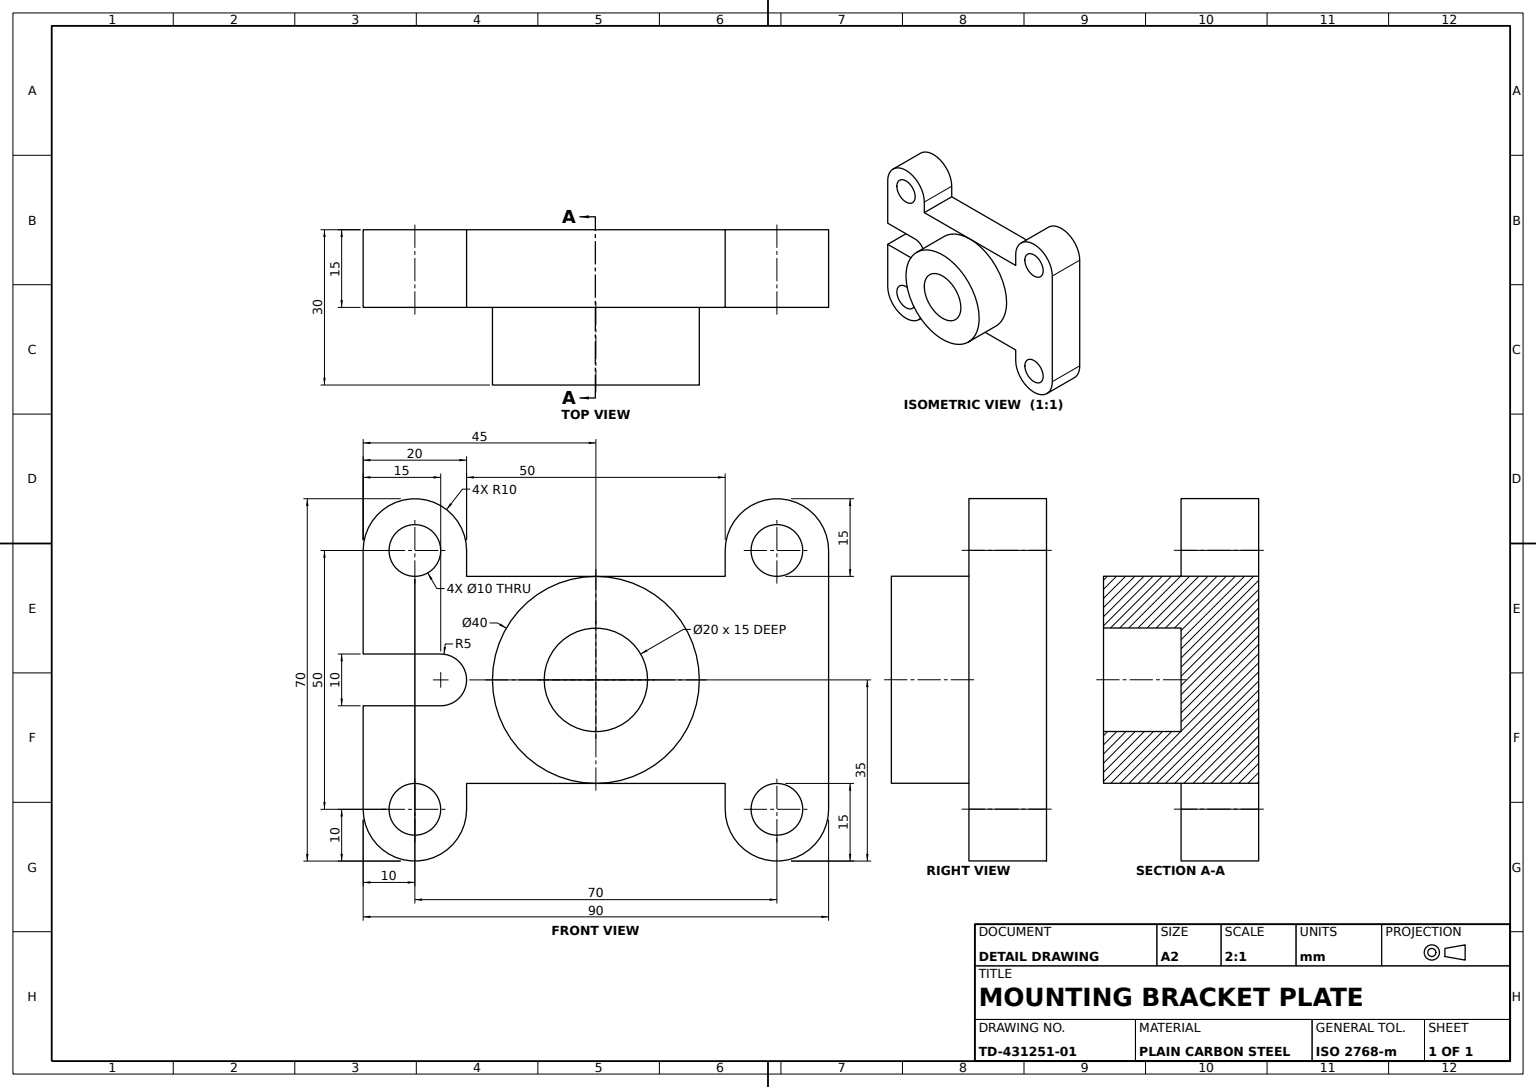
from build123d import *

# Parameters (mm, degrees)
BASE_PLATE_DEPTH           = 15
END_PAD_1_SKETCH_W         = 50
END_PAD_1_SKETCH_H         = 15
END_PAD_1_DEPTH            = 5
END_PAD_2_SKETCH_W         = 50
END_PAD_2_SKETCH_H         = 15
END_PAD_2_DEPTH            = 5
HUB_SKETCH_R               = 20
HUB_40_DEPTH               = 15
BORE_SKETCH_R              = 10
BORE_20_DEPTH              = 15
MOUNTING_HOLES_SKETCH_R    = 5
MOUNTING_HOLES_4X_10_DEPTH = 15
SIDE_NOTCH_DEPTH           = 15


with BuildPart() as part:
    # Base Plate Sketch → Base Plate (new body)
    with BuildSketch(Plane.XY):
        with BuildLine():
            Line((-10, 50), (-10, 0))
            ThreePointArc((-10, 0), (0, -10), (10, 0))
            Line((10, 0), (10, 10))
            Line((10, 10), (60, 10))
            Line((60, 10), (60, 0))
            ThreePointArc((60, 0), (70, -10), (80, 0))
            Line((80, 0), (80, 50))
            ThreePointArc((80, 50), (70, 60), (60, 50))
            Line((60, 50), (60, 40))
            Line((60, 40), (10, 40))
            Line((10, 40), (10, 50))
            ThreePointArc((10, 50), (0, 60), (-10, 50))
        make_face()
    extrude(amount=BASE_PLATE_DEPTH)

    # End Pad 1 Sketch → End Pad 1 (add)
    with BuildSketch(Plane(origin=(0, 40, 0), x_dir=(1, 0, 0), z_dir=(0, 1, 0))):
        with Locations((35, -7.5)):
            Rectangle(END_PAD_1_SKETCH_W, END_PAD_1_SKETCH_H)
    extrude(amount=END_PAD_1_DEPTH)

    # End Pad 2 Sketch → End Pad 2 (add)
    with BuildSketch(Plane.XZ.offset(-10)):
        with Locations((35, 7.5)):
            Rectangle(END_PAD_2_SKETCH_W, END_PAD_2_SKETCH_H)
    extrude(amount=END_PAD_2_DEPTH)

    # Hub Sketch → Hub Ø40 (add)
    with BuildSketch(Plane.XY.offset(15)):
        with Locations(Location((35, 25, 0), (0, 0, 270))):
            Circle(HUB_SKETCH_R)
    extrude(amount=HUB_40_DEPTH)

    # Bore Sketch → Bore Ø20 (cut)
    with BuildSketch(Plane.XY.offset(30)):
        with Locations((35, 25)):
            Circle(BORE_SKETCH_R)
    extrude(amount=-BORE_20_DEPTH, mode=Mode.SUBTRACT)

    # Mounting Holes Sketch → Mounting Holes 4xØ10 (cut)
    with BuildSketch(Plane.XY.offset(15)):
        with Locations((70, 50)):
            Circle(MOUNTING_HOLES_SKETCH_R)
        with Locations((70, 0)):
            Circle(MOUNTING_HOLES_SKETCH_R)
        Circle(MOUNTING_HOLES_SKETCH_R)
        with Locations((0, 50)):
            Circle(MOUNTING_HOLES_SKETCH_R)
    extrude(amount=-MOUNTING_HOLES_4X_10_DEPTH, mode=Mode.SUBTRACT)

    # Side Notch Sketch → Side Notch (cut)
    with BuildSketch(Plane.XY.offset(15)):
        with BuildLine():
            Line((-10, 30), (-10, 20))
            Line((-10, 20), (5, 20))
            ThreePointArc((5, 20), (10, 25), (5, 30))
            Line((5, 30), (-10, 30))
        make_face()
    extrude(amount=-SIDE_NOTCH_DEPTH, mode=Mode.SUBTRACT)


solid = part.part
